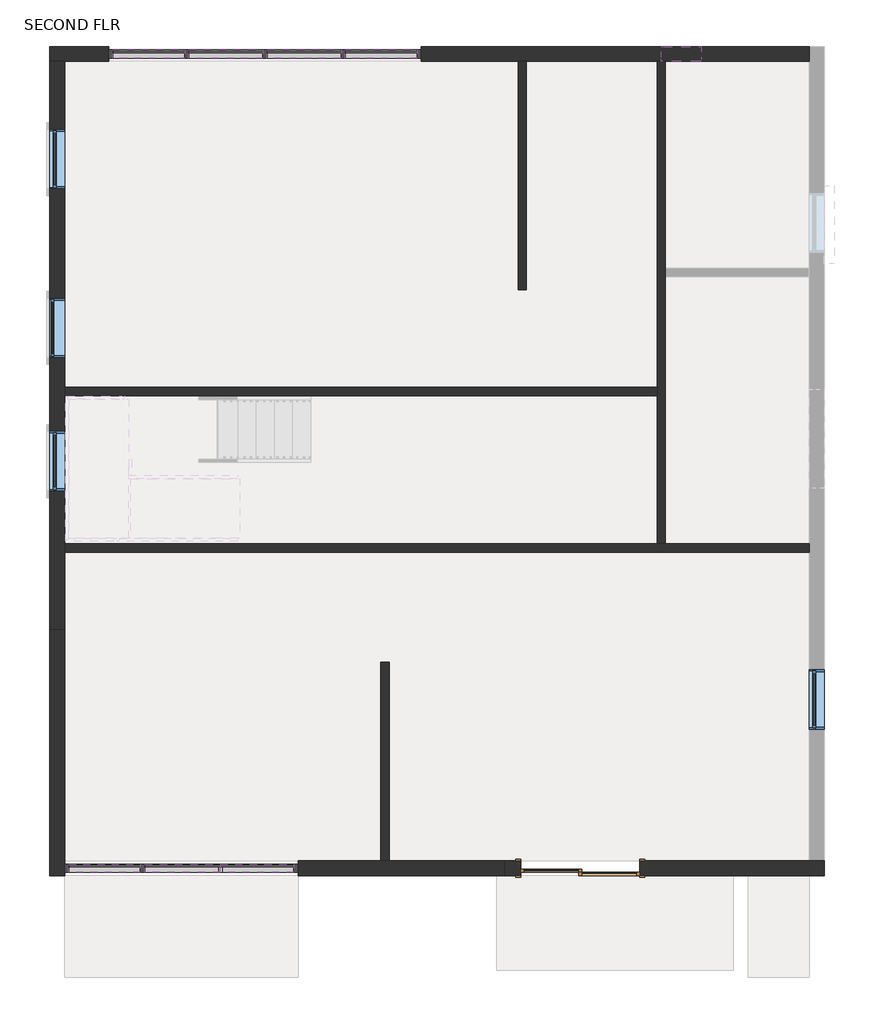
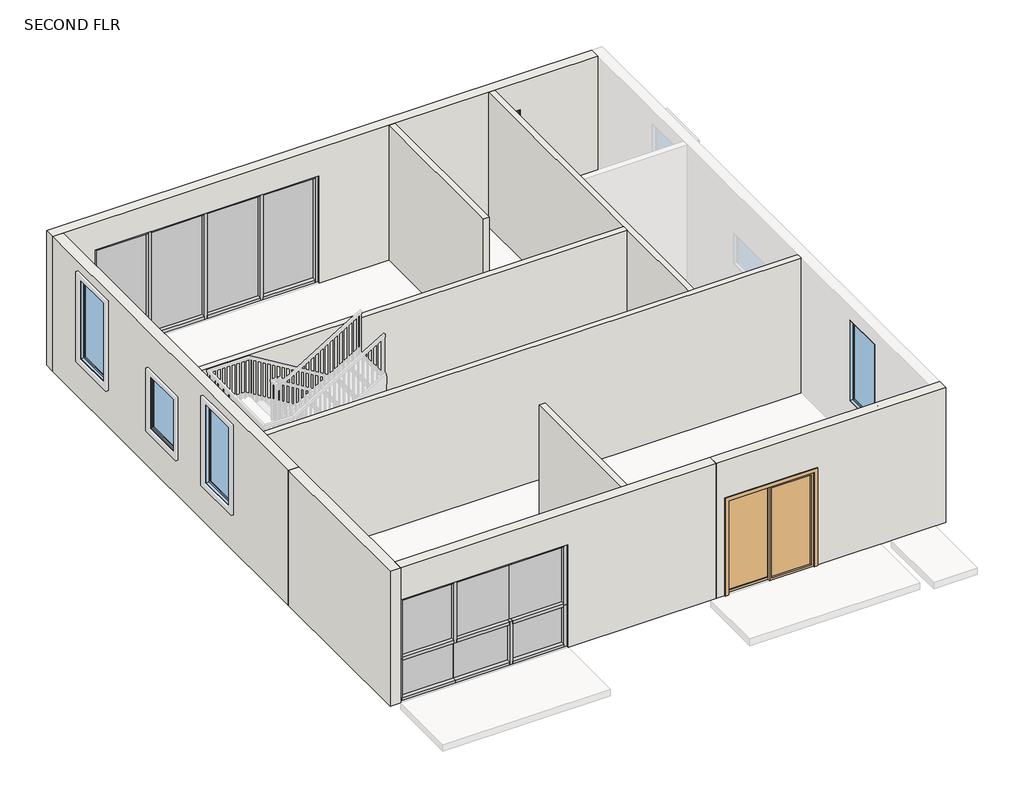
# One storey, part 1 of 3: 28 members, 11 walls, 10 plates, 5 windows, 1 door.
"""IFC4 building model written with IfcOpenShell, lengths in millimetres."""

from ifc_helpers import new_model, si_unit, frame, origin, place, context, project, spatial, polyline, outline, extrude, faceted_brep, transform, mapped, element, save
from components import door_d4d75d1e, member_37269937, member_65519335, member_c344cd1a, member_3285b992, member_e0b7b075, member_9e1336f4, member_4aea75b7, member_606b50d7, member_11090e01, member_d69c7880, member_a8685e1c, member_189d47d0, member_5afaafd3, system_panel_glazed_36bafcef, system_panel_glazed_3e9834e9, system_panel_glazed_4667a6f9, system_panel_glazed_1b898e97, system_panel_glazed_f332cf5d, system_panel_glazed_fcf423c9, system_panel_glazed_d43da186, system_panel_glazed_a1d10a75, window_80340324, window_c1f32544, window_2e8ca8a3

model = new_model("IFC4")

# Units and contexts
model_context = context("Model", 3, world=origin())
ifc_project = project(units=[si_unit("LENGTHUNIT", "METRE", prefix="MILLI")], contexts=[model_context])

# Site, building, storey
site = spatial("IfcSite", under=ifc_project)
building = spatial("IfcBuilding", under=site)
storey = spatial("IfcBuildingStorey", under=building, Name="SECOND FLR", Elevation=6400.8)

# Door
placement = place(None, origin())
door_shape = door_d4d75d1e(model_context)
element("IfcDoor", 1, ObjectType="Door-Double-Sliding : 72\" x 84\"", at=placement, inside=storey, context=model_context, shape_type="MappedRepresentation", body=[
    mapped(door_shape, transform((-1851.8781265, -4147.9142532, 6400.8), x_axis=(-1.0, 0.0, 0.0), y_axis=(0.0, -1.0, 0.0), z_axis=(0.0, 0.0, 1.0))),
])

# Members
member_shape = member_37269937(model_context)
element("IfcMember", 2, ObjectType="Rectangular Mullion : 2.5\" x 5\" rectangular", at=placement, inside=storey, context=model_context, shape_type="MappedRepresentation", body=[
    mapped(member_shape, transform((-8601.9281264, -4274.9142532, 8731.4935463), x_axis=(0.0, 0.0, 1.0), y_axis=(0.0, -1.0, 0.0), z_axis=(1.0, 0.0, 0.0))),
])
element("IfcMember", 3, ObjectType="Rectangular Mullion : 2.5\" x 5\" rectangular", at=placement, inside=storey, context=model_context, shape_type="MappedRepresentation", body=[
    mapped(member_shape, transform((-7344.6281266, -4274.9142532, 6400.8), x_axis=(0.0, 0.0, -1.0), y_axis=(0.0, -1.0, 0.0), z_axis=(-1.0, 0.0, 0.0))),
])
member_2_shape = member_65519335(model_context)
element("IfcMember", 4, ObjectType="Rectangular Mullion : 2.5\" x 5\" rectangular", at=placement, inside=storey, context=model_context, shape_type="MappedRepresentation", body=[
    mapped(member_2_shape, transform((-8601.9281264, -4274.9142532, 7343.5710507), x_axis=(0.0, 0.0, 1.0), y_axis=(0.0, -1.0, 0.0), z_axis=(1.0, 0.0, 0.0))),
])
element("IfcMember", 5, ObjectType="Rectangular Mullion : 2.5\" x 5\" rectangular", at=placement, inside=storey, context=model_context, shape_type="MappedRepresentation", body=[
    mapped(member_2_shape, transform((-6246.0781265, -4274.9142532, 7343.5710507), x_axis=(0.0, 0.0, 1.0), y_axis=(0.0, -1.0, 0.0), z_axis=(1.0, 0.0, 0.0))),
])
member_3_shape = member_c344cd1a(model_context)
element("IfcMember", 6, ObjectType="Rectangular Mullion : 2.5\" x 5\" rectangular", at=placement, inside=storey, context=model_context, shape_type="MappedRepresentation", body=[
    mapped(member_3_shape, transform((-7408.1281266, -4274.9142532, 7343.5710507), x_axis=(0.0, 0.0, 1.0), y_axis=(0.0, -1.0, 0.0), z_axis=(1.0, 0.0, 0.0))),
])
member_4_shape = member_3285b992(model_context)
element("IfcMember", 7, ObjectType="Rectangular Mullion : 2.5\" x 5\" rectangular", at=placement, inside=storey, context=model_context, shape_type="MappedRepresentation", body=[
    mapped(member_4_shape, transform((-9700.4781265, -4274.9142532, 6400.8), x_axis=(0.0, 0.0, -1.0), y_axis=(0.0, -1.0, 0.0), z_axis=(-1.0, 0.0, 0.0))),
])
member_5_shape = member_e0b7b075(model_context)
element("IfcMember", 8, ObjectType="Rectangular Mullion : 2.5\" x 5\" rectangular", at=placement, inside=storey, context=model_context, shape_type="MappedRepresentation", body=[
    mapped(member_5_shape, transform((-6182.5781265, -4274.9142532, 6400.8), x_axis=(1.0, 0.0, 0.0), y_axis=(0.0, -1.0, 0.0), z_axis=(0.0, 0.0, -1.0))),
])
element("IfcMember", 9, ObjectType="Rectangular Mullion : 2.5\" x 5\" rectangular", at=placement, inside=storey, context=model_context, shape_type="MappedRepresentation", body=[
    mapped(member_5_shape, transform((-9763.9781265, -4274.9142532, 7343.5710507), x_axis=(-1.0, 0.0, 0.0), y_axis=(0.0, -1.0, 0.0), z_axis=(0.0, 0.0, 1.0))),
])
member_6_shape = member_9e1336f4(model_context)
element("IfcMember", 10, ObjectType="Rectangular Mullion : 2.5\" x 5\" rectangular", at=placement, inside=storey, context=model_context, shape_type="MappedRepresentation", body=[
    mapped(member_6_shape, transform((-8570.1781264, -4274.9142532, 6400.8), x_axis=(0.0, 0.0, -1.0), y_axis=(0.0, -1.0, 0.0), z_axis=(-1.0, 0.0, 0.0))),
])
element("IfcMember", 11, ObjectType="Rectangular Mullion : 2.5\" x 5\" rectangular", at=placement, inside=storey, context=model_context, shape_type="MappedRepresentation", body=[
    mapped(member_4_shape, transform((-6246.0781265, -4274.9142532, 8731.4935463), x_axis=(0.0, 0.0, 1.0), y_axis=(0.0, -1.0, 0.0), z_axis=(1.0, 0.0, 0.0))),
])
element("IfcMember", 12, ObjectType="Rectangular Mullion : 2.5\" x 5\" rectangular", at=placement, inside=storey, context=model_context, shape_type="MappedRepresentation", body=[
    mapped(member_6_shape, transform((-7376.3781266, -4274.9142532, 8731.4935463), x_axis=(0.0, 0.0, 1.0), y_axis=(0.0, -1.0, 0.0), z_axis=(1.0, 0.0, 0.0))),
])
member_7_shape = member_4aea75b7(model_context)
element("IfcMember", 13, ObjectType="Rectangular Mullion : 2.5\" x 5\" rectangular", at=placement, inside=storey, context=model_context, shape_type="MappedRepresentation", body=[
    mapped(member_7_shape, transform((-7376.3781266, -4274.9142532, 6400.8), x_axis=(1.0, 0.0, 0.0), y_axis=(0.0, -1.0, 0.0), z_axis=(0.0, 0.0, -1.0))),
])
member_8_shape = member_606b50d7(model_context)
element("IfcMember", 14, ObjectType="Rectangular Mullion : 2.5\" x 5\" rectangular", at=placement, inside=storey, context=model_context, shape_type="MappedRepresentation", body=[
    mapped(member_8_shape, transform((-8570.1781264, -4274.9142532, 7311.8210507), x_axis=(1.0, 0.0, 0.0), y_axis=(0.0, -1.0, 0.0), z_axis=(0.0, 0.0, -1.0))),
])
member_9_shape = member_11090e01(model_context)
element("IfcMember", 15, ObjectType="Rectangular Mullion : 2.5\" x 5\" rectangular", at=placement, inside=storey, context=model_context, shape_type="MappedRepresentation", body=[
    mapped(member_9_shape, transform((-9763.9781265, -4274.9142532, 8731.4935463), x_axis=(-1.0, 0.0, 0.0), y_axis=(0.0, -1.0, 0.0), z_axis=(0.0, 0.0, 1.0))),
])
element("IfcMember", 16, ObjectType="Rectangular Mullion : 2.5\" x 5\" rectangular", at=placement, inside=storey, context=model_context, shape_type="MappedRepresentation", body=[
    mapped(member_9_shape, transform((-6182.5781265, -4274.9142532, 7343.5710507), x_axis=(1.0, 0.0, 0.0), y_axis=(0.0, -1.0, 0.0), z_axis=(0.0, 0.0, -1.0))),
])
member_10_shape = member_d69c7880(model_context)
element("IfcMember", 17, ObjectType="Rectangular Mullion : 2.5\" x 5\" rectangular", at=placement, inside=storey, context=model_context, shape_type="MappedRepresentation", body=[
    mapped(member_10_shape, transform((-4353.7781265, 8221.8857468, 8829.7640157), x_axis=(0.0, 0.0, 1.0), y_axis=(0.0, -1.0, 0.0), z_axis=(1.0, 0.0, 0.0))),
])
element("IfcMember", 18, ObjectType="Rectangular Mullion : 2.5\" x 5\" rectangular", at=placement, inside=storey, context=model_context, shape_type="MappedRepresentation", body=[
    mapped(member_10_shape, transform((-7922.4781263, 8221.8857468, 8829.7640157), x_axis=(0.0, 0.0, 1.0), y_axis=(0.0, -1.0, 0.0), z_axis=(1.0, 0.0, 0.0))),
])
member_11_shape = member_a8685e1c(model_context)
element("IfcMember", 19, ObjectType="Rectangular Mullion : 2.5\" x 5\" rectangular", at=placement, inside=storey, context=model_context, shape_type="MappedRepresentation", body=[
    mapped(member_11_shape, transform((-6722.3281265, 8221.8857468, 8829.7640157), x_axis=(0.0, 0.0, 1.0), y_axis=(0.0, -1.0, 0.0), z_axis=(1.0, 0.0, 0.0))),
])
element("IfcMember", 20, ObjectType="Rectangular Mullion : 2.5\" x 5\" rectangular", at=placement, inside=storey, context=model_context, shape_type="MappedRepresentation", body=[
    mapped(member_11_shape, transform((-5522.1781266, 8221.8857468, 8829.7640157), x_axis=(0.0, 0.0, 1.0), y_axis=(0.0, -1.0, 0.0), z_axis=(1.0, 0.0, 0.0))),
])
element("IfcMember", 21, ObjectType="Rectangular Mullion : 2.5\" x 5\" rectangular", at=placement, inside=storey, context=model_context, shape_type="MappedRepresentation", body=[
    mapped(member_10_shape, transform((-9027.3781265, 8221.8857468, 6400.8), x_axis=(0.0, 0.0, -1.0), y_axis=(0.0, -1.0, 0.0), z_axis=(-1.0, 0.0, 0.0))),
])
element("IfcMember", 22, ObjectType="Rectangular Mullion : 2.5\" x 5\" rectangular", at=placement, inside=storey, context=model_context, shape_type="MappedRepresentation", body=[
    mapped(member_10_shape, transform((-5458.6781266, 8221.8857468, 6400.8), x_axis=(0.0, 0.0, -1.0), y_axis=(0.0, -1.0, 0.0), z_axis=(-1.0, 0.0, 0.0))),
])
element("IfcMember", 23, ObjectType="Rectangular Mullion : 2.5\" x 5\" rectangular", at=placement, inside=storey, context=model_context, shape_type="MappedRepresentation", body=[
    mapped(member_11_shape, transform((-7858.9781263, 8221.8857468, 6400.8), x_axis=(0.0, 0.0, -1.0), y_axis=(0.0, -1.0, 0.0), z_axis=(-1.0, 0.0, 0.0))),
])
element("IfcMember", 24, ObjectType="Rectangular Mullion : 2.5\" x 5\" rectangular", at=placement, inside=storey, context=model_context, shape_type="MappedRepresentation", body=[
    mapped(member_11_shape, transform((-6658.8281265, 8221.8857468, 6400.8), x_axis=(0.0, 0.0, -1.0), y_axis=(0.0, -1.0, 0.0), z_axis=(-1.0, 0.0, 0.0))),
])
member_12_shape = member_189d47d0(model_context)
element("IfcMember", 25, ObjectType="Rectangular Mullion : 2.5\" x 5\" rectangular", at=placement, inside=storey, context=model_context, shape_type="MappedRepresentation", body=[
    mapped(member_12_shape, transform((-7890.7281263, 8221.8857468, 6400.8), x_axis=(1.0, 0.0, 0.0), y_axis=(0.0, -1.0, 0.0), z_axis=(0.0, 0.0, -1.0))),
])
element("IfcMember", 26, ObjectType="Rectangular Mullion : 2.5\" x 5\" rectangular", at=placement, inside=storey, context=model_context, shape_type="MappedRepresentation", body=[
    mapped(member_12_shape, transform((-6690.5781265, 8221.8857468, 6400.8), x_axis=(1.0, 0.0, 0.0), y_axis=(0.0, -1.0, 0.0), z_axis=(0.0, 0.0, -1.0))),
])
element("IfcMember", 27, ObjectType="Rectangular Mullion : 2.5\" x 5\" rectangular", at=placement, inside=storey, context=model_context, shape_type="MappedRepresentation", body=[
    mapped(member_12_shape, transform((-5490.4281266, 8221.8857468, 6400.8), x_axis=(1.0, 0.0, 0.0), y_axis=(0.0, -1.0, 0.0), z_axis=(0.0, 0.0, -1.0))),
])
member_13_shape = member_5afaafd3(model_context)
element("IfcMember", 28, ObjectType="Rectangular Mullion : 2.5\" x 5\" rectangular", at=placement, inside=storey, context=model_context, shape_type="MappedRepresentation", body=[
    mapped(member_13_shape, transform((-4290.2781265, 8221.8857468, 6400.8), x_axis=(1.0, 0.0, 0.0), y_axis=(0.0, -1.0, 0.0), z_axis=(0.0, 0.0, -1.0))),
])
element("IfcMember", 29, ObjectType="Rectangular Mullion : 2.5\" x 5\" rectangular", at=placement, inside=storey, context=model_context, shape_type="MappedRepresentation", body=[
    mapped(member_13_shape, transform((-9090.8781265, 8221.8857468, 8829.7640157), x_axis=(-1.0, 0.0, 0.0), y_axis=(0.0, -1.0, 0.0), z_axis=(0.0, 0.0, 1.0))),
])

# Plates
system_panel_glazed_shape = system_panel_glazed_36bafcef(model_context)
element("IfcPlate", 30, ObjectType="System Panel : Glazed", at=placement, inside=storey, context=model_context, shape_type="MappedRepresentation", body=[
    mapped(system_panel_glazed_shape, transform((-9135.3281264, -4274.9142532, 6464.3), x_axis=(1.0, 0.0, 0.0), y_axis=(0.0, 1.0, 0.0), z_axis=(0.0, 0.0, 1.0))),
])
system_panel_glazed_2_shape = system_panel_glazed_3e9834e9(model_context)
element("IfcPlate", 31, ObjectType="System Panel : Glazed", at=placement, inside=storey, context=model_context, shape_type="MappedRepresentation", body=[
    mapped(system_panel_glazed_2_shape, transform((-7989.1531265, -4274.9142532, 6464.3), x_axis=(1.0, 0.0, 0.0), y_axis=(0.0, 1.0, 0.0), z_axis=(0.0, 0.0, 1.0))),
])
system_panel_glazed_3_shape = system_panel_glazed_4667a6f9(model_context)
element("IfcPlate", 32, ObjectType="System Panel : Glazed", at=placement, inside=storey, context=model_context, shape_type="MappedRepresentation", body=[
    mapped(system_panel_glazed_3_shape, transform((-6795.3531265, -4274.9142532, 6464.3), x_axis=(1.0, 0.0, 0.0), y_axis=(0.0, 1.0, 0.0), z_axis=(0.0, 0.0, 1.0))),
])
system_panel_glazed_4_shape = system_panel_glazed_1b898e97(model_context)
element("IfcPlate", 33, ObjectType="System Panel : Glazed", at=placement, inside=storey, context=model_context, shape_type="MappedRepresentation", body=[
    mapped(system_panel_glazed_4_shape, transform((-9151.2031264, -4274.9142532, 7375.3210507), x_axis=(1.0, 0.0, 0.0), y_axis=(0.0, 1.0, 0.0), z_axis=(0.0, 0.0, 1.0))),
])
system_panel_glazed_5_shape = system_panel_glazed_f332cf5d(model_context)
element("IfcPlate", 34, ObjectType="System Panel : Glazed", at=placement, inside=storey, context=model_context, shape_type="MappedRepresentation", body=[
    mapped(system_panel_glazed_5_shape, transform((-7957.4031265, -4274.9142532, 7375.3210507), x_axis=(1.0, 0.0, 0.0), y_axis=(0.0, 1.0, 0.0), z_axis=(0.0, 0.0, 1.0))),
])
system_panel_glazed_6_shape = system_panel_glazed_fcf423c9(model_context)
element("IfcPlate", 35, ObjectType="System Panel : Glazed", at=placement, inside=storey, context=model_context, shape_type="MappedRepresentation", body=[
    mapped(system_panel_glazed_6_shape, transform((-6811.2281265, -4274.9142532, 7375.3210507), x_axis=(1.0, 0.0, 0.0), y_axis=(0.0, 1.0, 0.0), z_axis=(0.0, 0.0, 1.0))),
])
system_panel_glazed_7_shape = system_panel_glazed_d43da186(model_context)
element("IfcPlate", 36, ObjectType="System Panel : Glazed", at=placement, inside=storey, context=model_context, shape_type="MappedRepresentation", body=[
    mapped(system_panel_glazed_7_shape, transform((-8474.9281264, 8221.8857468, 6464.3), x_axis=(1.0, 0.0, 0.0), y_axis=(0.0, 1.0, 0.0), z_axis=(0.0, 0.0, 1.0))),
])
element("IfcPlate", 37, ObjectType="System Panel : Glazed", at=placement, inside=storey, context=model_context, shape_type="MappedRepresentation", body=[
    mapped(system_panel_glazed_7_shape, transform((-4906.2281265, 8221.8857468, 6464.3), x_axis=(1.0, 0.0, 0.0), y_axis=(0.0, 1.0, 0.0), z_axis=(0.0, 0.0, 1.0))),
])
system_panel_glazed_8_shape = system_panel_glazed_a1d10a75(model_context)
element("IfcPlate", 38, ObjectType="System Panel : Glazed", at=placement, inside=storey, context=model_context, shape_type="MappedRepresentation", body=[
    mapped(system_panel_glazed_8_shape, transform((-7290.6531264, 8221.8857468, 6464.3), x_axis=(1.0, 0.0, 0.0), y_axis=(0.0, 1.0, 0.0), z_axis=(0.0, 0.0, 1.0))),
])
element("IfcPlate", 39, ObjectType="System Panel : Glazed", at=placement, inside=storey, context=model_context, shape_type="MappedRepresentation", body=[
    mapped(system_panel_glazed_8_shape, transform((-6090.5031265, 8221.8857468, 6464.3), x_axis=(1.0, 0.0, 0.0), y_axis=(0.0, 1.0, 0.0), z_axis=(0.0, 0.0, 1.0))),
])

# Walls
element("IfcWall", 40, ObjectType="INNER WALL THICKNESS 5\"", at=placement, inside=storey, context=model_context, shape_type="SweptSolid", body=[
    extrude(outline(polyline([(-9763.9781265, 3103.7857468), (-670.7781265, 3103.7857468), (-670.7781265, 2976.7857468), (-9763.9781265, 2976.7857468), (-9763.9781265, 3103.7857468)])), frame((0.0, 0.0, 6400.8), z_axis=(0.0, 0.0, 1.0), x_axis=(1.0, 0.0, 0.0)), (0.0, 0.0, 1.0), 3048.0),
])
element("IfcWall", 41, ObjectType="INNER WALL THICKNESS 5\"", at=placement, inside=storey, context=model_context, shape_type="Brep", body=[
    faceted_brep([(1666.0218735, 703.1165128, 6400.8), (-543.7781265, 703.1165128, 6400.8), (-670.7781265, 703.1165128, 6400.8), (-9763.9781265, 703.1165128, 6400.8), (-9763.9781265, 703.1165128, 9448.8), (-670.7781265, 703.1165128, 9448.8), (-543.7781265, 703.1165128, 9448.8), (1666.0218735, 703.1165128, 9448.8), (1666.0218735, 576.1165128, 6400.8), (1666.0218735, 576.1165128, 9448.8), (-9763.9781265, 576.1165128, 9448.8), (-9763.9781265, 576.1165128, 6400.8)], [[[0, 1, 2, 3, 4, 5, 6, 7]], [[8, 9, 10, 11]], [[3, 2, 1, 0, 8, 11]], [[7, 6, 5, 4, 10, 9]], [[0, 7, 9, 8]], [[4, 3, 11, 10]]]),
])
element("IfcWall", 42, ObjectType="INNER WALL THICKNESS 5\"", at=placement, inside=storey, context=model_context, shape_type="Brep", body=[
    faceted_brep([(-543.7781265, 703.1165128, 6400.8), (-543.7781265, 4805.5857468, 6400.8), (-543.7781265, 4932.5857468, 6400.8), (-543.7781265, 8107.5857468, 6400.8), (-543.7781265, 8107.5857468, 9448.8), (-543.7781265, 4932.5857468, 9448.8), (-543.7781265, 4805.5857468, 9448.8), (-543.7781265, 703.1165128, 9448.8), (-670.7781265, 703.1165128, 6400.8), (-670.7781265, 703.1165128, 9448.8), (-670.7781265, 2976.7857468, 9448.8), (-670.7781265, 3103.7857468, 9448.8), (-670.7781265, 8107.5857468, 9448.8), (-670.7781265, 8107.5857468, 6400.8), (-670.7781265, 3103.7857468, 6400.8), (-670.7781265, 2976.7857468, 6400.8)], [[[0, 1, 2, 3, 4, 5, 6, 7]], [[8, 9, 10, 11, 12, 13, 14, 15]], [[3, 2, 1, 0, 8, 15, 14, 13]], [[7, 6, 5, 4, 12, 11, 10, 9]], [[0, 7, 9, 8]], [[4, 3, 13, 12]]]),
])
element("IfcWall", 43, ObjectType="INNER WALL THICKNESS 5\"", at=placement, inside=storey, context=model_context, shape_type="SweptSolid", body=[
    extrude(outline(polyline([(-2804.3781265, 4602.3857468), (-2804.3781265, 8107.5857468), (-2677.3781265, 8107.5857468), (-2677.3781265, 4602.3857468), (-2804.3781265, 4602.3857468)])), frame((0.0, 0.0, 6400.8), z_axis=(0.0, 0.0, 1.0), x_axis=(1.0, 0.0, 0.0)), (0.0, 0.0, 1.0), 3048.0),
])
element("IfcWall", 44, ObjectType="INNER WALL THICKNESS 5\"", at=placement, inside=storey, context=model_context, shape_type="SweptSolid", body=[
    extrude(outline(polyline([(-4785.5781265, -1112.6142532), (-4785.5781265, -4160.6142532), (-4912.5781265, -4160.6142532), (-4912.5781265, -1112.6142532), (-4785.5781265, -1112.6142532)])), frame((0.0, 0.0, 6400.8), z_axis=(0.0, 0.0, 1.0), x_axis=(1.0, 0.0, 0.0)), (0.0, 0.0, 1.0), 3048.0),
])
element("IfcWall", 45, ObjectType="OUTER WALL THICKNESS 9\"", at=placement, inside=storey, context=model_context, shape_type="Brep", body=[
    faceted_brep([(1894.6218735, -4389.2142532, 9448.8), (-3020.2781265, -4389.2142532, 9448.8), (-3020.2781265, -4389.2142532, 6400.8), (-2766.2781265, -4389.2142532, 6400.8), (-2766.2781265, -4389.2142532, 8534.4), (-937.4781265, -4389.2142532, 8534.4), (-937.4781265, -4389.2142532, 6400.8), (1894.6218735, -4389.2142532, 6400.8), (-3020.2781265, -4160.6142532, 9448.8), (1666.0218735, -4160.6142532, 9448.8), (1894.6218735, -4160.6142532, 9448.8), (1894.6218735, -4160.6142532, 6400.8), (1666.0218735, -4160.6142532, 6400.8), (-937.4781265, -4160.6142532, 6400.8), (-937.4781265, -4160.6142532, 8534.4), (-2766.2781265, -4160.6142532, 8534.4), (-2766.2781265, -4160.6142532, 6400.8), (-3020.2781265, -4160.6142532, 6400.8)], [[[0, 1, 2, 3, 4, 5, 6, 7]], [[8, 9, 10, 11, 12, 13, 14, 15, 16, 17]], [[11, 7, 6, 13, 12]], [[2, 17, 16, 3]], [[1, 0, 10, 9, 8]], [[2, 1, 8, 17]], [[0, 7, 11, 10]], [[5, 14, 13, 6]], [[14, 5, 4, 15]], [[15, 4, 3, 16]]]),
])
element("IfcWall", 46, ObjectType="OUTER WALL THICKNESS 9\"", at=placement, inside=storey, context=model_context, shape_type="Brep", body=[
    faceted_brep([(-9992.5781265, 8336.1857468, 9448.8), (1666.0218735, 8336.1857468, 9448.8), (1666.0218735, 8336.1857468, 6400.8), (-4290.2781265, 8336.1857468, 6400.8), (-4290.2781265, 8336.1857468, 8829.7640157), (-9090.8781265, 8336.1857468, 8829.7640157), (-9090.8781265, 8336.1857468, 6400.8), (-9992.5781265, 8336.1857468, 6400.8), (-607.2781265, 8336.1857468, 8822.5330034), (-607.2781265, 8336.1857468, 8212.9330034), (2.3218735, 8336.1857468, 8212.9330034), (2.3218735, 8336.1857468, 8822.5330034), (1666.0218735, 8107.5857468, 9448.8), (-543.7781265, 8107.5857468, 9448.8), (-670.7781265, 8107.5857468, 9448.8), (-2677.3781265, 8107.5857468, 9448.8), (-2804.3781265, 8107.5857468, 9448.8), (-9763.9781265, 8107.5857468, 9448.8), (-9992.5781265, 8107.5857468, 9448.8), (-9992.5781265, 8107.5857468, 6400.8), (-9763.9781265, 8107.5857468, 6400.8), (-9090.8781265, 8107.5857468, 6400.8), (-9090.8781265, 8107.5857468, 8829.7640157), (-4290.2781265, 8107.5857468, 8829.7640157), (-4290.2781265, 8107.5857468, 6400.8), (-2804.3781265, 8107.5857468, 6400.8), (-2677.3781265, 8107.5857468, 6400.8), (-670.7781265, 8107.5857468, 6400.8), (-543.7781265, 8107.5857468, 6400.8), (1666.0218735, 8107.5857468, 6400.8), (-607.2781265, 8107.5857468, 8822.5330034), (2.3218735, 8107.5857468, 8822.5330034), (2.3218735, 8107.5857468, 8212.9330034), (-607.2781265, 8107.5857468, 8212.9330034)], [[[0, 1, 2, 3, 4, 5, 6, 7], [8, 9, 10, 11]], [[12, 13, 14, 15, 16, 17, 18, 19, 20, 21, 22, 23, 24, 25, 26, 27, 28, 29], [30, 31, 32, 33]], [[2, 29, 28, 27, 26, 25, 24, 3]], [[19, 7, 6, 21, 20]], [[1, 0, 18, 17, 16, 15, 14, 13, 12]], [[2, 1, 12, 29]], [[0, 7, 19, 18]], [[5, 22, 21, 6]], [[22, 5, 4, 23]], [[23, 4, 3, 24]], [[9, 8, 30, 33]], [[10, 9, 33, 32]], [[11, 10, 32, 31]], [[8, 11, 31, 30]]]),
])
element("IfcWall", 47, ObjectType="OUTER WALL THICKNESS 9\"", at=placement, inside=storey, context=model_context, shape_type="Brep", body=[
    faceted_brep([(-9992.5781265, 8107.5857468, 6400.8), (-9992.5781265, -617.3142532, 6400.8), (-9992.5781265, -617.3142532, 9448.8), (-9992.5781265, 8107.5857468, 9448.8), (-9992.5781265, 7066.1857468, 9144.0), (-9992.5781265, 6151.7857468, 9144.0), (-9992.5781265, 6151.7857468, 7315.2), (-9992.5781265, 7066.1857468, 7315.2), (-9992.5781265, 2430.6857468, 9144.0), (-9992.5781265, 1516.2857468, 9144.0), (-9992.5781265, 1516.2857468, 7315.2), (-9992.5781265, 2430.6857468, 7315.2), (-9992.5781265, 4475.3857468, 8534.4), (-9992.5781265, 3560.9857468, 8534.4), (-9992.5781265, 3560.9857468, 7315.2), (-9992.5781265, 4475.3857468, 7315.2), (-9763.9781265, 8107.5857468, 6400.8), (-9763.9781265, 8107.5857468, 9448.8), (-9763.9781265, 3103.7857468, 9448.8), (-9763.9781265, 2976.7857468, 9448.8), (-9763.9781265, 703.1165128, 9448.8), (-9763.9781265, 576.1165128, 9448.8), (-9763.9781265, -617.3142532, 9448.8), (-9763.9781265, -617.3142532, 6400.8), (-9763.9781265, 576.1165128, 6400.8), (-9763.9781265, 703.1165128, 6400.8), (-9763.9781265, 2976.7857468, 6400.8), (-9763.9781265, 3103.7857468, 6400.8), (-9763.9781265, 7066.1857468, 9144.0), (-9763.9781265, 7066.1857468, 7315.2), (-9763.9781265, 6151.7857468, 7315.2), (-9763.9781265, 6151.7857468, 9144.0), (-9763.9781265, 2430.6857468, 9144.0), (-9763.9781265, 2430.6857468, 7315.2), (-9763.9781265, 1516.2857468, 7315.2), (-9763.9781265, 1516.2857468, 9144.0), (-9763.9781265, 4475.3857468, 8534.4), (-9763.9781265, 4475.3857468, 7315.2), (-9763.9781265, 3560.9857468, 7315.2), (-9763.9781265, 3560.9857468, 8534.4)], [[[0, 1, 2, 3], [4, 5, 6, 7], [8, 9, 10, 11], [12, 13, 14, 15]], [[16, 17, 18, 19, 20, 21, 22, 23, 24, 25, 26, 27], [28, 29, 30, 31], [32, 33, 34, 35], [36, 37, 38, 39]], [[1, 0, 16, 27, 26, 25, 24, 23]], [[2, 1, 23, 22]], [[3, 2, 22, 21, 20, 19, 18, 17]], [[0, 3, 17, 16]], [[29, 28, 4, 7]], [[30, 29, 7, 6]], [[31, 30, 6, 5]], [[28, 31, 5, 4]], [[33, 32, 8, 11]], [[34, 33, 11, 10]], [[35, 34, 10, 9]], [[32, 35, 9, 8]], [[37, 36, 12, 15]], [[38, 37, 15, 14]], [[39, 38, 14, 13]], [[36, 39, 13, 12]]]),
])
element("IfcWall", 48, ObjectType="OUTER WALL THICKNESS 9\"", at=placement, inside=storey, context=model_context, shape_type="Brep", body=[
    faceted_brep([(-9992.5781265, -617.3142532, 6400.8), (-9992.5781265, -4389.2142532, 6400.8), (-9992.5781265, -4389.2142532, 9448.8), (-9992.5781265, -617.3142532, 9448.8), (-9763.9781265, -617.3142532, 6400.8), (-9763.9781265, -617.3142532, 9448.8), (-9763.9781265, -4160.6142532, 9448.8), (-9763.9781265, -4389.2142532, 9448.8), (-9763.9781265, -4389.2142532, 9229.1131521), (-9763.9781265, -4389.2142532, 6400.8)], [[[0, 1, 2, 3]], [[4, 5, 6, 7, 8, 9]], [[1, 0, 4, 9]], [[3, 2, 7, 6, 5]], [[0, 3, 5, 4]], [[2, 1, 9, 8, 7]]]),
])
element("IfcWall", 49, ObjectType="OUTER WALL THICKNESS 9\"", at=placement, inside=storey, context=model_context, shape_type="Brep", body=[
    faceted_brep([(-3020.2781265, -4389.2142532, 6400.8), (-3020.2781265, -4389.2142532, 9448.8), (-9763.9781265, -4389.2142532, 9448.8), (-9763.9781265, -4389.2142532, 8731.4935463), (-6182.5781265, -4389.2142532, 8731.4935463), (-6182.5781265, -4389.2142532, 6400.8), (-3020.2781265, -4160.6142532, 9448.8), (-3020.2781265, -4160.6142532, 6400.8), (-4785.5781265, -4160.6142532, 6400.8), (-4912.5781265, -4160.6142532, 6400.8), (-6182.5781265, -4160.6142532, 6400.8), (-6182.5781265, -4160.6142532, 8731.4935463), (-9763.9781265, -4160.6142532, 8731.4935463), (-9763.9781265, -4160.6142532, 9448.8), (-4912.5781265, -4160.6142532, 9448.8), (-4785.5781265, -4160.6142532, 9448.8)], [[[0, 1, 2, 3, 4, 5]], [[6, 7, 8, 9, 10, 11, 12, 13, 14, 15]], [[7, 0, 5, 10, 9, 8]], [[1, 0, 7, 6]], [[2, 1, 6, 15, 14, 13]], [[2, 13, 12, 3]], [[11, 4, 3, 12]], [[4, 11, 10, 5]]]),
])
element("IfcWall", 50, ObjectType="OUTER WALL THICKNESS 9\"", at=placement, inside=storey, context=model_context, shape_type="SweptSolid", body=[
    extrude(outline(polyline([(497.6218735, -4300.3142532), (497.6218735, -4274.9142532), (726.2218735, -4274.9142532), (726.2218735, -4300.3142532), (497.6218735, -4300.3142532)])), frame((0.0, 0.0, 6400.8), z_axis=(0.0, 0.0, 1.0), x_axis=(1.0, 0.0, 0.0)), (0.0, 0.0, 1.0), 3048.0),
])

# Windows
window_shape = window_80340324(model_context)
element("IfcWindow", 51, ObjectType="Fixed : 24\" x 24\"", at=placement, inside=storey, context=model_context, shape_type="MappedRepresentation", body=[
    mapped(window_shape, transform((-340.5781265, 8221.8857468, 7298.5330034), x_axis=(-1.0, 0.0, 0.0), y_axis=(0.0, -1.0, 0.0), z_axis=(0.0, 0.0, 1.0))),
])
window_2_shape = window_c1f32544(model_context)
element("IfcWindow", 52, ObjectType="Fixed : 36\" x 48\"", at=placement, inside=storey, context=model_context, shape_type="MappedRepresentation", body=[
    mapped(window_2_shape, transform((-9878.2781265, 4056.2857468, 6400.8), x_axis=(0.0, 1.0, 0.0), y_axis=(-1.0, 0.0, 0.0), z_axis=(0.0, 0.0, 1.0))),
])
window_3_shape = window_2e8ca8a3(model_context)
element("IfcWindow", 53, ObjectType="Fixed : window 3' x 6\"", at=placement, inside=storey, context=model_context, shape_type="MappedRepresentation", body=[
    mapped(window_3_shape, transform((1780.3218735, -1646.0142532, 6400.8), x_axis=(0.0, 1.0, 0.0), y_axis=(-1.0, 0.0, 0.0), z_axis=(0.0, 0.0, 1.0))),
])
element("IfcWindow", 54, ObjectType="Fixed : window 3' x 6\"", at=placement, inside=storey, context=model_context, shape_type="MappedRepresentation", body=[
    mapped(window_3_shape, transform((-9878.2781265, 6647.0857468, 6400.8), x_axis=(0.0, 1.0, 0.0), y_axis=(-1.0, 0.0, 0.0), z_axis=(0.0, 0.0, 1.0))),
])
element("IfcWindow", 55, ObjectType="Fixed : window 3' x 6\"", at=placement, inside=storey, context=model_context, shape_type="MappedRepresentation", body=[
    mapped(window_3_shape, transform((-9878.2781265, 2011.5857468, 6400.8), x_axis=(0.0, 1.0, 0.0), y_axis=(-1.0, 0.0, 0.0), z_axis=(0.0, 0.0, 1.0))),
])

save(model, "model.ifc")

# Revit data of these elements
# Type "Door-Double-Sliding : 72\" x 84\""
#   Type Mark = "8"
#   Construction Type Id = "opn-d45"
#   Assembly Code = "C1020"
#   Analytic Construction = "Wood frame, double glass door "
#   Thickness = 0' - 2"
#   Thermal Resistance (R) = 1.8150 (h·ft²·°F)/BTU
#   Heat Transfer Coefficient (U) = 0.5510 BTU/(h·ft²·°F)
#   Height = 7' - 0"
#   Rail Width = 0' - 2"
#   Stiles = 0' - 2"
#   Trim Projection Ext = 0' - 1"
#   Trim Projection Int = 0' - 1"
#   Trim Width = 0' - 3"
#   Width = 6' - 0"
#   Define Thermal Properties by = 1
#   Glazing = Glass
#   Panel Material = Wood - Birch - Solid Stained Light Low Gloss
#   Trim Material = Paint - Sienna
#   Visual Light Transmittance = 0
#   Solar Heat Gain Coefficient = 0
#   Function = (empty or 0)
#   Wall Closure = (empty or 0)
# Type "Rectangular Mullion : 2.5\" x 5\" rectangular"
#   built-in parameter 1007304 = 0.416667 (stored number, unit not read)
#   built-in parameter 1007301 = 0.104167 (stored number, unit not read)
#   built-in parameter 1007300 = 0.104167 (stored number, unit not read)
# Type "System Panel : Glazed"
#   Construction Type Id = "GSP4R"
#   Analytic Construction = "1/8 in Pilkington single glazing"
#   Visual Light Transmittance = 0.9
#   Solar Heat Gain Coefficient = 0.86
#   Heat Transfer Coefficient (U) = 1.18115 BTU/(h·ft²·°F)
#   Define Thermal Properties by = 1
# Type "INNER WALL THICKNESS 5\""
#   Assembly Code = "B2010"
#   Layers, outside or top first: 0' - 5" "WALL PAINT" (function 1)
# Type "OUTER WALL THICKNESS 9\""
#   Assembly Code = "B2010"
#   Layers, outside or top first: 0' - 9" "WALL PAINT" (function 1)
# Type "Fixed : 24\" x 24\""
#   Type Mark = "3"
#   Construction Type Id = "GSP4R"
#   Assembly Code = "B2020100"
#   Analytic Construction = "1/8 in Pilkington single glazing"
#   Visual Light Transmittance = 0.9
#   Solar Heat Gain Coefficient = 0.78
#   Heat Transfer Coefficient (U) = 0.6496 BTU/(h·ft²·°F)
#   Height = 2' - 0"
#   Default Sill Height = 3' - 0"
#   Width = 2' - 0"
#   Window Inset = 0' - 0 3/4"
#   Define Thermal Properties by = 1
#   Define Thermal Properties by = 1
#   Glass Pane Material = Glass
#   Sash Material = Sash
#   Wall Closure = (empty or 0)
# Type "Fixed : 36\" x 48\""
#   Type Mark = "1"
#   Construction Type Id = "GSP4R"
#   Assembly Code = "B2020100"
#   Analytic Construction = "1/8 in Pilkington single glazing"
#   Visual Light Transmittance = 0.9
#   Solar Heat Gain Coefficient = 0.78
#   Heat Transfer Coefficient (U) = 0.6496 BTU/(h·ft²·°F)
#   Height = 4' - 0"
#   Default Sill Height = 3' - 0"
#   Width = 3' - 0"
#   Window Inset = 0' - 0 3/4"
#   Define Thermal Properties by = 1
#   Define Thermal Properties by = 1
#   Glass Pane Material = Glass
#   Sash Material = Sash
#   Wall Closure = (empty or 0)
# Type "Fixed : window 3' x 6\""
#   Type Mark = "26"
#   Construction Type Id = "GSP4R"
#   Assembly Code = "B2020100"
#   Analytic Construction = "1/8 in Pilkington single glazing"
#   Visual Light Transmittance = 0.9
#   Solar Heat Gain Coefficient = 0.78
#   Heat Transfer Coefficient (U) = 0.6496 BTU/(h·ft²·°F)
#   Height = 6' - 0"
#   Default Sill Height = 3' - 0"
#   Width = 3' - 0"
#   Window Inset = 0' - 2"
#   Define Thermal Properties by = 1
#   Glass Pane Material = Glass
#   Sash Material = Sash
#   Wall Closure = (empty or 0)
# Element 1 (IfcDoor, "Door-Double-Sliding : 72\" x 84\"")
#   Phase Created = New Construction
#   Materials on its faces: "Paint - Sienna", "Wood - Birch - Solid Stained Light Low Gloss", "Glass"
# Elements 2, 3, 4, 5, 6, 7, 8, 9, 10, 11, 12, 13, 14, 15, 16, 17, 18, 19, 20, 21, 22, 23, 24, 25, 26, 27, 28, 29 (IfcMember, "Rectangular Mullion : 2.5\" x 5\" rectangular")
#   Phase Created = New Construction
#   Materials on its faces: "BLACK COLOUR"
# Elements 30, 31, 32, 33, 34, 35, 36, 37, 38, 39 (IfcPlate, "System Panel : Glazed")
#   Phase Created = New Construction
#   Materials on its faces: "Glass"
# Element 40 (IfcWall, "INNER WALL THICKNESS 5\"")
#   Top Offset = 10' - 0"
#   Base Offset = 0' - 0"
#   wall height = 10' - 0"
#   Phase Created = New Construction
#   Base Constraint = SECOND FLR
#   Top Constraint = SECOND FLR
#   Materials on its faces: "WALL PAINT"
# Elements 41, 42, 43, 44 (IfcWall, "INNER WALL THICKNESS 5\"")
#   Top Offset = 0' - 0"
#   Base Offset = 0' - 0"
#   Unconnected Height = 10' - 0"
#   wall height = 10' - 0"
#   Phase Created = New Construction
#   Base Constraint = SECOND FLR
#   Materials on its faces: "WALL PAINT"
# Elements 45, 46, 48, 49, 50 (IfcWall, "OUTER WALL THICKNESS 9\"")
#   Top Offset = 0' - 0"
#   Base Offset = 0' - 0"
#   Unconnected Height = 10' - 0"
#   wall height = 10' - 0"
#   Phase Created = New Construction
#   Base Constraint = SECOND FLR
#   Materials on its faces: "WALL PAINT"
# Element 47 (IfcWall, "OUTER WALL THICKNESS 9\"")
#   Top Offset = 10' - 0"
#   Base Offset = 0' - 0"
#   wall height = 10' - 0"
#   Phase Created = New Construction
#   Base Constraint = SECOND FLR
#   Top Constraint = SECOND FLR
#   Materials on its faces: "WALL PAINT"
# Element 51 (IfcWindow, "Fixed : 24\" x 24\"")
#   Mark = "29"
#   Phase Created = New Construction
#   Materials on its faces: "Sash", "Glass"
# Element 52 (IfcWindow, "Fixed : 36\" x 48\"")
#   Mark = "26"
#   Phase Created = New Construction
#   Materials on its faces: "Sash", "Glass"
# Element 53 (IfcWindow, "Fixed : window 3' x 6\"")
#   Mark = "11"
#   Phase Created = New Construction
#   Materials on its faces: "Sash", "Glass"
# Element 54 (IfcWindow, "Fixed : window 3' x 6\"")
#   Mark = "22"
#   Phase Created = New Construction
#   Materials on its faces: "Sash", "Glass"
# Element 55 (IfcWindow, "Fixed : window 3' x 6\"")
#   Mark = "24"
#   Phase Created = New Construction
#   Materials on its faces: "Sash", "Glass"
# Materials
#   "Glass": class "Glass", colour RGB 0 128 192, transparency 0.75, Description = "Soda Lime Glass", Cost = 0
#   "Wood - Birch - Solid Stained Light Low Gloss": class "Wood", colour RGB 210 159 95, transparency 0, Cost = 0
#   "Paint - Sienna": colour RGB 118 70 51, transparency 0, Cost = 0
#   "WALL PAINT": class "Generic", colour RGB 120 120 120, transparency 0, Cost = 0
#   "Sash": class "Wood", colour RGB 224 178 126, transparency 0, Cost = 0
#   "BLACK COLOUR": class "Generic", colour RGB 120 120 120, transparency 0, Cost = 0
# Room at (-5242.778, 1839.951) mm, phase "New Construction", upper level "SECOND FLR", upper offset 10' - 0", lower offset 0' - 0"
#   Number = "14"
#   Name = "STAIRS ROOM"
# Room at (586.522, 6545.486) mm, phase "New Construction", upper level "SECOND FLR", upper offset 10' - 0", lower offset 0' - 0"
#   Number = "15"
#   Name = "TOILET"
# Room at (586.522, 2754.351) mm, phase "New Construction", upper level "SECOND FLR", upper offset 10' - 0", lower offset 0' - 0"
#   Number = "16"
#   Name = "TOILET"
# Room at (-5242.778, 5631.086) mm, phase "New Construction", upper level "SECOND FLR", upper offset 10' - 0", lower offset 0' - 0"
#   Number = "17"
#   Name = "BEDROOM AND STUDY ROOM"
# Room at (-4048.978, -1817.649) mm, phase "New Construction", upper level "SECOND FLR", upper offset 10' - 0", lower offset 0' - 0"
#   Number = "18"
#   Name = "BEDROOM AND STUDY ROOM"
